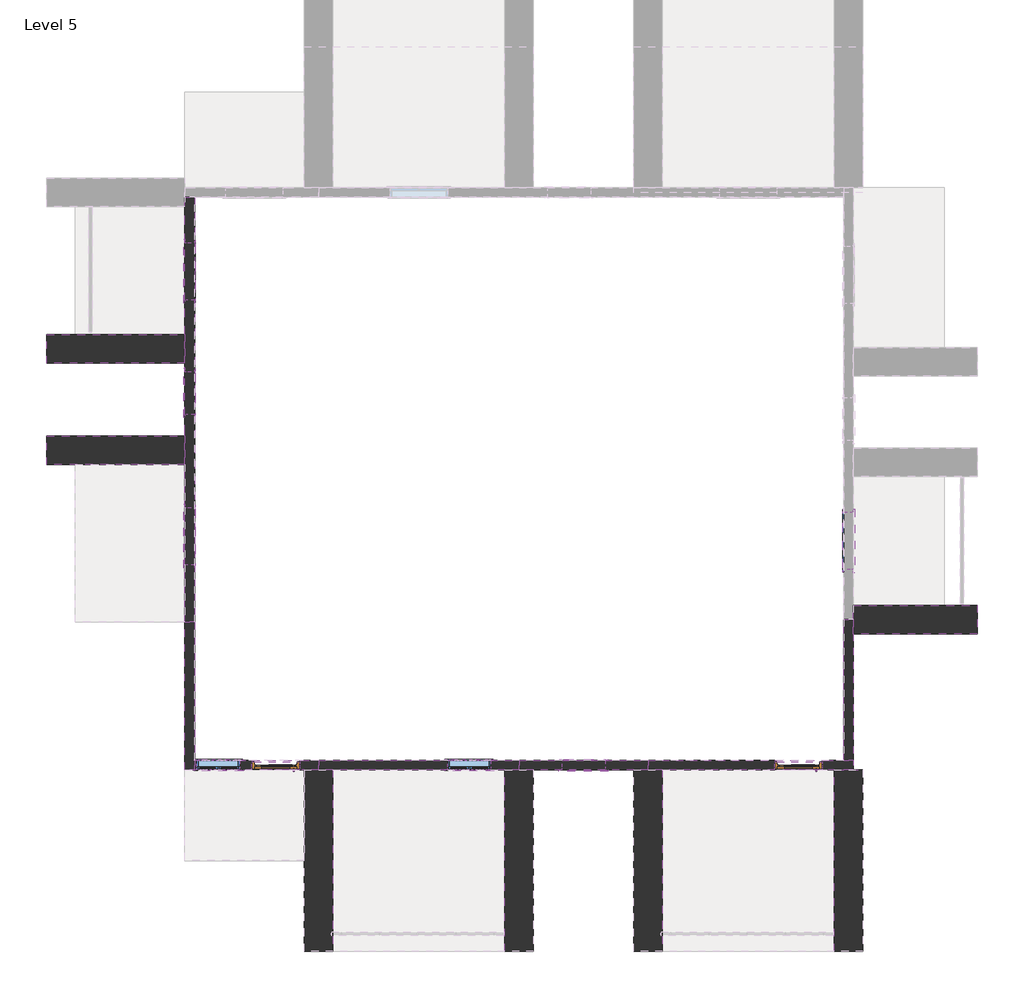
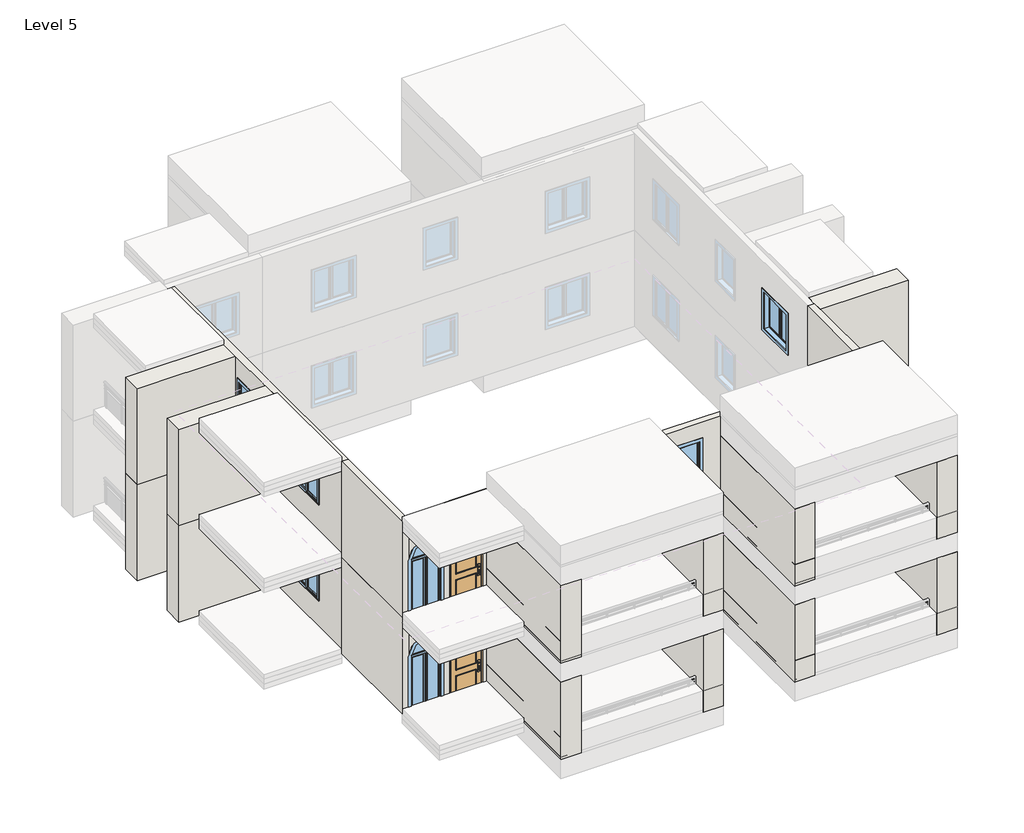
# One storey, part 1 of 4: 28 walls, 14 windows, 4 doors.
"""IFC4 building model written with IfcOpenShell, lengths in millimetres."""

from ifc_helpers import new_model, si_unit, frame, origin, place, context, project, spatial, polyline, circle_curve, outline, extrude, faceted_brep, transform, mapped, element, save
from ifc_brep_helpers import plane_surface, revolved_surface, advanced_brep
from components import door_b6c2ee01, window_4e95f2a8, window_0862ab64, window_8a4441b2

model = new_model("IFC4")

# Units and contexts
model_context = context("Model", 3, world=origin())
ifc_project = project(units=[si_unit("LENGTHUNIT", "METRE", prefix="MILLI")], contexts=[model_context])

# Site, building, storey
site = spatial("IfcSite", under=ifc_project)
building = spatial("IfcBuilding", under=site)
storey = spatial("IfcBuildingStorey", under=building, Name="Level 5", Elevation=12192.0)

# Doors
placement = place(None, origin())
door_shape = door_b6c2ee01(model_context)
element("IfcDoor", 1, ObjectType="Door-Exterior-Single-Two_Lite : 36\" x 94\"", at=placement, inside=storey, context=model_context, shape_type="MappedRepresentation", body=[
    mapped(door_shape, transform((-10452.2937431, -5765.036389, 12192.0), x_axis=(-1.0, 0.0, 0.0), y_axis=(0.0, -1.0, 0.0), z_axis=(0.0, 0.0, 1.0))),
])
element("IfcDoor", 2, ObjectType="Door-Exterior-Single-Two_Lite : 36\" x 94\"", at=placement, inside=storey, context=model_context, shape_type="MappedRepresentation", body=[
    mapped(door_shape, transform((672.9062569, -5765.036389, 12192.0), x_axis=(-1.0, 0.0, 0.0), y_axis=(0.0, -1.0, 0.0), z_axis=(0.0, 0.0, 1.0))),
])
element("IfcDoor", 3, ObjectType="Door-Exterior-Single-Two_Lite : 36\" x 94\"", at=placement, inside=storey, context=model_context, shape_type="MappedRepresentation", body=[
    mapped(door_shape, transform((-10452.2937431, -5765.036389, 15240.0), x_axis=(-1.0, 0.0, 0.0), y_axis=(0.0, -1.0, 0.0), z_axis=(0.0, 0.0, 1.0))),
])
element("IfcDoor", 4, ObjectType="Door-Exterior-Single-Two_Lite : 36\" x 94\"", at=placement, inside=storey, context=model_context, shape_type="MappedRepresentation", body=[
    mapped(door_shape, transform((672.9062569, -5765.036389, 15240.0), x_axis=(-1.0, 0.0, 0.0), y_axis=(0.0, -1.0, 0.0), z_axis=(0.0, 0.0, 1.0))),
])

# Walls
element("IfcWall", 5, ObjectType="Generic - 8\"", at=placement, inside=storey, context=model_context, shape_type="Brep", body=[
    faceted_brep([(-12179.4937431, -5872.986389, 12496.8), (-12179.4937431, -5669.786389, 12496.8), (-12179.4937431, -2723.386389, 12496.8), (-12179.4937431, -2723.386389, 15544.8), (-12179.4937431, -5669.786389, 15544.8), (-12179.4937431, -5872.986389, 15544.8), (-12382.6937431, -5872.986389, 12496.8), (-12382.6937431, -5872.986389, 15544.8), (-12382.6937431, -2723.386389, 15544.8), (-12382.6937431, -2723.386389, 12496.8)], [[[0, 1, 2, 3, 4, 5]], [[6, 7, 8, 9]], [[2, 1, 0, 6, 9]], [[3, 2, 9, 8]], [[5, 4, 3, 8, 7]], [[0, 5, 7, 6]]]),
])
element("IfcWall", 6, ObjectType="Generic - 8\"", at=placement, inside=storey, context=model_context, shape_type="Brep", body=[
    faceted_brep([(-2527.4937431, -5669.786389, 15544.8), (1638.1062569, -5669.786389, 15544.8), (1841.3062569, -5669.786389, 15544.8), (1841.3062569, -5669.786389, 12496.8), (1638.1062569, -5669.786389, 12496.8), (1180.9062569, -5669.786389, 12496.8), (1180.9062569, -5669.786389, 14681.2), (164.9062569, -5669.786389, 14681.2), (164.9062569, -5669.786389, 12496.8), (-2527.4937431, -5669.786389, 12496.8), (1841.3062569, -5872.986389, 15544.8), (-2527.4937431, -5872.986389, 15544.8), (-2527.4937431, -5872.986389, 12496.8), (-2222.6937431, -5872.986389, 12496.8), (164.9062569, -5872.986389, 12496.8), (164.9062569, -5872.986389, 14681.2), (1180.9062569, -5872.986389, 14681.2), (1180.9062569, -5872.986389, 12496.8), (1434.9062569, -5872.986389, 12496.8), (1841.3062569, -5872.986389, 12496.8)], [[[0, 1, 2, 3, 4, 5, 6, 7, 8, 9]], [[10, 11, 12, 13, 14, 15, 16, 17, 18, 19]], [[3, 19, 18, 17, 5, 4]], [[12, 9, 8, 14, 13]], [[2, 1, 0, 11, 10]], [[2, 10, 19, 3]], [[7, 15, 14, 8]], [[15, 7, 6, 16]], [[16, 6, 5, 17]], [[9, 12, 11, 0]]]),
])
element("IfcWall", 7, ObjectType="Generic - 8\"", at=placement, inside=storey, context=model_context, shape_type="Brep", body=[
    faceted_brep([(-12179.4937431, -2723.386389, 12496.8), (-12179.4937431, 6319.013611, 12496.8), (-12179.4937431, 6319.013611, 15544.8), (-12179.4937431, -2723.386389, 15544.8), (-12179.4937431, 2610.613611, 14867.7149116), (-12179.4937431, 2610.613611, 13648.5149116), (-12179.4937431, 1696.213611, 13648.5149116), (-12179.4937431, 1696.213611, 14867.7149116), (-12179.4937431, -284.986389, 14690.8059909), (-12179.4937431, -284.986389, 13471.6059909), (-12179.4937431, -1504.186389, 13471.6059909), (-12179.4937431, -1504.186389, 14690.8059909), (-12179.4937431, 5353.813611, 14617.1335827), (-12179.4937431, 5353.813611, 13397.9335827), (-12179.4937431, 4134.613611, 13397.9335827), (-12179.4937431, 4134.613611, 14617.1335827), (-12382.6937431, -2723.386389, 12496.8), (-12382.6937431, -2723.386389, 15544.8), (-12382.6937431, 629.413611, 15544.8), (-12382.6937431, 1239.013611, 15544.8), (-12382.6937431, 2788.413611, 15544.8), (-12382.6937431, 3398.013611, 15544.8), (-12382.6937431, 6115.813611, 15544.8), (-12382.6937431, 6319.013611, 15544.8), (-12382.6937431, 6319.013611, 12496.8), (-12382.6937431, 6115.813611, 12496.8), (-12382.6937431, 3398.013611, 12496.8), (-12382.6937431, 2788.413611, 12496.8), (-12382.6937431, 1239.013611, 12496.8), (-12382.6937431, 629.413611, 12496.8), (-12382.6937431, 2610.613611, 14867.7149116), (-12382.6937431, 1696.213611, 14867.7149116), (-12382.6937431, 1696.213611, 13648.5149116), (-12382.6937431, 2610.613611, 13648.5149116), (-12382.6937431, -284.986389, 14690.8059909), (-12382.6937431, -1504.186389, 14690.8059909), (-12382.6937431, -1504.186389, 13471.6059909), (-12382.6937431, -284.986389, 13471.6059909), (-12382.6937431, 5353.813611, 14617.1335827), (-12382.6937431, 4134.613611, 14617.1335827), (-12382.6937431, 4134.613611, 13397.9335827), (-12382.6937431, 5353.813611, 13397.9335827)], [[[0, 1, 2, 3], [4, 5, 6, 7], [8, 9, 10, 11], [12, 13, 14, 15]], [[16, 17, 18, 19, 20, 21, 22, 23, 24, 25, 26, 27, 28, 29], [30, 31, 32, 33], [34, 35, 36, 37], [38, 39, 40, 41]], [[1, 0, 16, 29, 28, 27, 26, 25, 24]], [[3, 2, 23, 22, 21, 20, 19, 18, 17]], [[0, 3, 17, 16]], [[2, 1, 24, 23]], [[5, 4, 30, 33]], [[6, 5, 33, 32]], [[7, 6, 32, 31]], [[4, 7, 31, 30]], [[9, 8, 34, 37]], [[10, 9, 37, 36]], [[11, 10, 36, 35]], [[8, 11, 35, 34]], [[13, 12, 38, 41]], [[14, 13, 41, 40]], [[15, 14, 40, 39]], [[12, 15, 39, 38]]]),
])
element("IfcWall", 8, ObjectType="Generic - 8\"", at=placement, inside=storey, context=model_context, shape_type="AdvancedBrep", body=[
    advanced_brep(
    [(-12179.4937431, -5669.786389, 15544.8), (-9537.8937431, -5669.786389, 15544.8), (-9537.8937431, -5669.786389, 12496.8), (-9944.2937431, -5669.786389, 12496.8), (-9944.2937431, -5669.786389, 14681.2), (-10960.2937431, -5669.786389, 14681.2), (-10960.2937431, -5669.786389, 12496.8), (-11214.2937431, -5669.786389, 12496.8), (-11214.2937431, -5669.786389, 14235.597687), (-12128.6937431, -5669.786389, 14235.597687), (-12128.6937431, -5669.786389, 12496.8), (-12179.4937431, -5669.786389, 12496.8), (-9537.8937431, -5872.986389, 15544.8), (-12179.4937431, -5872.986389, 15544.8), (-12179.4937431, -5872.986389, 12496.8), (-12128.6937431, -5872.986389, 12496.8), (-12128.6937431, -5872.986389, 14235.597687), (-11214.2937431, -5872.986389, 14235.597687), (-11214.2937431, -5872.986389, 12496.8), (-10960.2937431, -5872.986389, 12496.8), (-10960.2937431, -5872.986389, 14681.2), (-9944.2937431, -5872.986389, 14681.2), (-9944.2937431, -5872.986389, 12496.8), (-9842.6937431, -5872.986389, 12496.8), (-9537.8937431, -5872.986389, 12496.8)],
    [
        (0, 1),
        (1, 2),
        (2, 3),
        (3, 4),
        (4, 5),
        (5, 6),
        (6, 7),
        (7, 8),
        (8, 9, circle_curve(frame((-11671.4937431, -5669.786389, 14235.597687), z_axis=(0.0, -1.0, 0.0), x_axis=(-1.0, 0.0, 0.0)), 457.2)),
        (9, 10),
        (10, 11),
        (11, 0),
        (12, 13),
        (13, 14),
        (14, 15),
        (15, 16),
        (16, 17, circle_curve(frame((-11671.4937431, -5872.986389, 14235.597687), z_axis=(0.0, 1.0, 0.0), x_axis=(-1.0, 0.0, 0.0)), 457.2)),
        (17, 18),
        (18, 19),
        (19, 20),
        (20, 21),
        (21, 22),
        (22, 23),
        (23, 24),
        (24, 12),
        (14, 11),
        (10, 15),
        (2, 24),
        (22, 3),
        (6, 19),
        (18, 7),
        (0, 13),
        (12, 1),
        (5, 20),
        (4, 21),
        (9, 16),
        (17, 8),
    ],
    [
        plane_surface(frame((1423.3958892, -5669.786389, 12496.8), z_axis=(0.0, 1.0, 0.0), x_axis=(-1.0, 0.0, 0.0))),
        plane_surface(frame((1423.3958892, -5872.986389, 12496.8), z_axis=(0.0, -1.0, 0.0), x_axis=(1.0, 0.0, 0.0))),
        plane_surface(frame((-9537.8937431, -5669.786389, 12496.8), z_axis=(0.0, 0.0, -1.0), x_axis=(0.0, -1.0, 0.0))),
        plane_surface(frame((-12281.0937431, -5669.786389, 15544.8), z_axis=(0.0, 0.0, 1.0), x_axis=(0.0, -1.0, 0.0))),
        plane_surface(frame((-12179.4937431, 6416.9740134, 12496.8), z_axis=(-1.0, 0.0, 0.0), x_axis=(0.0, 1.0, 0.0))),
        plane_surface(frame((-9537.8937431, -5669.786389, 15544.8), z_axis=(1.0, 0.0, 0.0), x_axis=(0.0, -1.0, 0.0))),
        plane_surface(frame((-10960.2937431, -4145.786389, 12192.0), z_axis=(1.0, 0.0, 0.0), x_axis=(0.0, -1.0, 0.0))),
        plane_surface(frame((-10960.2937431, -4145.786389, 14681.2), z_axis=(0.0, 0.0, -1.0), x_axis=(0.0, -1.0, 0.0))),
        plane_surface(frame((-9944.2937431, -4145.786389, 14681.2), z_axis=(-1.0, 0.0, 0.0), x_axis=(0.0, -1.0, 0.0))),
        plane_surface(frame((-12128.6937431, -7193.786389, 14235.597687), z_axis=(1.0, 0.0, 0.0), x_axis=(0.0, 1.0, 0.0))),
        plane_surface(frame((-11214.2937431, -7193.786389, 12387.747687), z_axis=(-1.0, 0.0, 0.0), x_axis=(0.0, 1.0, 0.0))),
        revolved_surface(polyline([(-12128.6937431, -5872.986389, 14235.597687), (-12128.6937431, -5669.786389, 14235.597687)]), (-11671.4937431, -4145.786389, 14235.597687), (0.0, -1.0, 0.0)),
    ],
    [
        (0, [[1, 2, 3, 4, 5, 6, 7, 8, 9, 10, 11, 12]]),
        (1, [[13, 14, 15, 16, 17, 18, 19, 20, 21, 22, 23, 24, 25]]),
        (2, [[26, -11, 27, -15]]),
        (2, [[28, -24, -23, 29, -3]]),
        (2, [[30, -19, 31, -7]]),
        (3, [[-1, 32, -13, 33]]),
        (4, [[-12, -26, -14, -32]]),
        (5, [[-33, -25, -28, -2]]),
        (6, [[34, -20, -30, -6]]),
        (7, [[-34, -5, 35, -21]]),
        (8, [[-35, -4, -29, -22]]),
        (9, [[36, -16, -27, -10]]),
        (10, [[37, -8, -31, -18]]),
        (11, [[-36, -9, -37, -17]]),
    ],
),
])
element("IfcWall", 9, ObjectType="Generic - 8\"", at=placement, inside=storey, context=model_context, shape_type="Brep", body=[
    faceted_brep([(1638.1062569, -2672.586389, 12496.8), (1638.1062569, -5669.786389, 12496.8), (1638.1062569, -5669.786389, 15544.8), (1638.1062569, -2672.586389, 15544.8), (1841.3062569, -2672.586389, 12496.8), (1841.3062569, -2672.586389, 15544.8), (1841.3062569, -2977.386389, 15544.8), (1841.3062569, -5669.786389, 15544.8), (1841.3062569, -5669.786389, 12496.8), (1841.3062569, -2977.386389, 12496.8)], [[[0, 1, 2, 3]], [[4, 5, 6, 7, 8, 9]], [[1, 0, 4, 9, 8]], [[3, 2, 7, 6, 5]], [[0, 3, 5, 4]], [[1, 8, 7, 2]]]),
])
element("IfcWall", 10, ObjectType="Generic - 8\"", at=placement, inside=storey, context=model_context, shape_type="Brep", body=[
    faceted_brep([(-2527.4937431, -5669.786389, 15544.8), (-2527.4937431, -5669.786389, 12496.8), (-5270.6937431, -5669.786389, 12496.8), (-5270.6937431, -5669.786389, 15544.8), (-4356.2937431, -5669.786389, 14991.074951), (-4356.2937431, -5669.786389, 13771.874951), (-3441.8937431, -5669.786389, 13771.874951), (-3441.8937431, -5669.786389, 14991.074951), (-2527.4937431, -5872.986389, 12496.8), (-2527.4937431, -5872.986389, 15544.8), (-5270.6937431, -5872.986389, 15544.8), (-5270.6937431, -5872.986389, 12496.8), (-4965.8937431, -5872.986389, 12496.8), (-2832.2937431, -5872.986389, 12496.8), (-4356.2937431, -5872.986389, 14991.074951), (-3441.8937431, -5872.986389, 14991.074951), (-3441.8937431, -5872.986389, 13771.874951), (-4356.2937431, -5872.986389, 13771.874951)], [[[0, 1, 2, 3], [4, 5, 6, 7]], [[8, 9, 10, 11, 12, 13], [14, 15, 16, 17]], [[2, 1, 8, 13, 12, 11]], [[0, 3, 10, 9]], [[5, 4, 14, 17]], [[6, 5, 17, 16]], [[7, 6, 16, 15]], [[4, 7, 15, 14]], [[0, 9, 8, 1]], [[2, 11, 10, 3]]]),
])
element("IfcWall", 11, ObjectType="Generic - 8\"", at=placement, inside=storey, context=model_context, shape_type="AdvancedBrep", body=[
    advanced_brep(
    [(-9537.8937431, -5669.786389, 15544.8), (-5270.6937431, -5669.786389, 15544.8), (-5270.6937431, -5669.786389, 12496.8), (-5880.2937431, -5669.786389, 12496.8), (-5880.2937431, -5669.786389, 14192.25), (-6794.6937431, -5669.786389, 14192.25), (-6794.6937431, -5669.786389, 12496.8), (-9537.8937431, -5669.786389, 12496.8), (-5270.6937431, -5872.986389, 15544.8), (-9537.8937431, -5872.986389, 15544.8), (-9537.8937431, -5872.986389, 12496.8), (-9233.0937431, -5872.986389, 12496.8), (-6794.6937431, -5872.986389, 12496.8), (-6794.6937431, -5872.986389, 14192.25), (-5880.2937431, -5872.986389, 14192.25), (-5880.2937431, -5872.986389, 12496.8), (-5575.4937431, -5872.986389, 12496.8), (-5270.6937431, -5872.986389, 12496.8)],
    [
        (0, 1),
        (1, 2),
        (2, 3),
        (3, 4),
        (4, 5, circle_curve(frame((-6337.4937431, -5669.786389, 14192.25), z_axis=(0.0, -1.0, 0.0), x_axis=(-1.0, 0.0, 0.0)), 457.2)),
        (5, 6),
        (6, 7),
        (7, 0),
        (8, 9),
        (9, 10),
        (10, 11),
        (11, 12),
        (12, 13),
        (13, 14, circle_curve(frame((-6337.4937431, -5872.986389, 14192.25), z_axis=(0.0, 1.0, 0.0), x_axis=(-1.0, 0.0, 0.0)), 457.2)),
        (14, 15),
        (15, 16),
        (16, 17),
        (17, 8),
        (10, 7),
        (6, 12),
        (2, 17),
        (15, 3),
        (0, 9),
        (8, 1),
        (5, 13),
        (14, 4),
    ],
    [
        plane_surface(frame((1423.3958892, -5669.786389, 12496.8), z_axis=(0.0, 1.0, 0.0), x_axis=(-1.0, 0.0, 0.0))),
        plane_surface(frame((1423.3958892, -5872.986389, 12496.8), z_axis=(0.0, -1.0, 0.0), x_axis=(1.0, 0.0, 0.0))),
        plane_surface(frame((-5270.6937431, -5669.786389, 12496.8), z_axis=(0.0, 0.0, -1.0), x_axis=(0.0, -1.0, 0.0))),
        plane_surface(frame((-9537.8937431, -5669.786389, 15544.8), z_axis=(0.0, 0.0, 1.0), x_axis=(0.0, -1.0, 0.0))),
        plane_surface(frame((-6794.6937431, -7193.786389, 14192.25), z_axis=(1.0, 0.0, 0.0), x_axis=(0.0, 1.0, 0.0))),
        plane_surface(frame((-5880.2937431, -7193.786389, 12344.4), z_axis=(-1.0, 0.0, 0.0), x_axis=(0.0, 1.0, 0.0))),
        revolved_surface(polyline([(-6794.6937431, -5872.986389, 14192.25), (-6794.6937431, -5669.786389, 14192.25)]), (-6337.4937431, -4145.786389, 14192.25), (0.0, -1.0, 0.0)),
        plane_surface(frame((-5270.6937431, -5669.786389, 15544.8), z_axis=(1.0, 0.0, 0.0), x_axis=(0.0, -1.0, 0.0))),
        plane_surface(frame((-9537.8937431, -5669.786389, 12496.8), z_axis=(-1.0, 0.0, 0.0), x_axis=(0.0, -1.0, 0.0))),
    ],
    [
        (0, [[1, 2, 3, 4, 5, 6, 7, 8]]),
        (1, [[9, 10, 11, 12, 13, 14, 15, 16, 17, 18]]),
        (2, [[19, -7, 20, -12, -11]]),
        (2, [[21, -17, -16, 22, -3]]),
        (3, [[-1, 23, -9, 24]]),
        (4, [[25, -13, -20, -6]]),
        (5, [[26, -4, -22, -15]]),
        (6, [[-25, -5, -26, -14]]),
        (7, [[-24, -18, -21, -2]]),
        (8, [[-19, -10, -23, -8]]),
    ],
),
])
element("IfcWall", 12, ObjectType="Generic - 8\"", at=placement, inside=storey, context=model_context, shape_type="Brep", body=[
    faceted_brep([(-12179.4937431, -5872.986389, 15544.8), (-12179.4937431, -5669.786389, 15544.8), (-12179.4937431, -2723.386389, 15544.8), (-12179.4937431, -2723.386389, 18592.8), (-12179.4937431, -5669.786389, 18592.8), (-12179.4937431, -5872.986389, 18592.8), (-12382.6937431, -5872.986389, 15544.8), (-12382.6937431, -5872.986389, 18592.8), (-12382.6937431, -2723.386389, 18592.8), (-12382.6937431, -2723.386389, 15544.8)], [[[0, 1, 2, 3, 4, 5]], [[6, 7, 8, 9]], [[2, 1, 0, 6, 9]], [[3, 2, 9, 8]], [[5, 4, 3, 8, 7]], [[0, 5, 7, 6]]]),
])
element("IfcWall", 13, ObjectType="Generic - 8\"", at=placement, inside=storey, context=model_context, shape_type="Brep", body=[
    faceted_brep([(-2527.4937431, -5669.786389, 18592.8), (1638.1062569, -5669.786389, 18592.8), (1841.3062569, -5669.786389, 18592.8), (1841.3062569, -5669.786389, 15544.8), (1638.1062569, -5669.786389, 15544.8), (1180.9062569, -5669.786389, 15544.8), (1180.9062569, -5669.786389, 17729.2), (164.9062569, -5669.786389, 17729.2), (164.9062569, -5669.786389, 15544.8), (-2527.4937431, -5669.786389, 15544.8), (1841.3062569, -5872.986389, 18592.8), (-2527.4937431, -5872.986389, 18592.8), (-2527.4937431, -5872.986389, 15544.8), (-2222.6937431, -5872.986389, 15544.8), (164.9062569, -5872.986389, 15544.8), (164.9062569, -5872.986389, 17729.2), (1180.9062569, -5872.986389, 17729.2), (1180.9062569, -5872.986389, 15544.8), (1434.9062569, -5872.986389, 15544.8), (1841.3062569, -5872.986389, 15544.8)], [[[0, 1, 2, 3, 4, 5, 6, 7, 8, 9]], [[10, 11, 12, 13, 14, 15, 16, 17, 18, 19]], [[3, 19, 18, 17, 5, 4]], [[12, 9, 8, 14, 13]], [[2, 1, 0, 11, 10]], [[2, 10, 19, 3]], [[7, 15, 14, 8]], [[15, 7, 6, 16]], [[16, 6, 5, 17]], [[9, 12, 11, 0]]]),
])
element("IfcWall", 14, ObjectType="Generic - 8\"", at=placement, inside=storey, context=model_context, shape_type="Brep", body=[
    faceted_brep([(-12179.4937431, -2723.386389, 15544.8), (-12179.4937431, 6319.013611, 15544.8), (-12179.4937431, 6319.013611, 18592.8), (-12179.4937431, -2723.386389, 18592.8), (-12179.4937431, 2610.613611, 17915.7149116), (-12179.4937431, 2610.613611, 16696.5149116), (-12179.4937431, 1696.213611, 16696.5149116), (-12179.4937431, 1696.213611, 17915.7149116), (-12179.4937431, -284.986389, 17738.8059909), (-12179.4937431, -284.986389, 16519.6059909), (-12179.4937431, -1504.186389, 16519.6059909), (-12179.4937431, -1504.186389, 17738.8059909), (-12179.4937431, 5353.813611, 17665.1335827), (-12179.4937431, 5353.813611, 16445.9335827), (-12179.4937431, 4134.613611, 16445.9335827), (-12179.4937431, 4134.613611, 17665.1335827), (-12382.6937431, -2723.386389, 15544.8), (-12382.6937431, -2723.386389, 18592.8), (-12382.6937431, 629.413611, 18592.8), (-12382.6937431, 1239.013611, 18592.8), (-12382.6937431, 2788.413611, 18592.8), (-12382.6937431, 3398.013611, 18592.8), (-12382.6937431, 6115.813611, 18592.8), (-12382.6937431, 6319.013611, 18592.8), (-12382.6937431, 6319.013611, 15544.8), (-12382.6937431, 6115.813611, 15544.8), (-12382.6937431, 3398.013611, 15544.8), (-12382.6937431, 2788.413611, 15544.8), (-12382.6937431, 1239.013611, 15544.8), (-12382.6937431, 629.413611, 15544.8), (-12382.6937431, 2610.613611, 17915.7149116), (-12382.6937431, 1696.213611, 17915.7149116), (-12382.6937431, 1696.213611, 16696.5149116), (-12382.6937431, 2610.613611, 16696.5149116), (-12382.6937431, -284.986389, 17738.8059909), (-12382.6937431, -1504.186389, 17738.8059909), (-12382.6937431, -1504.186389, 16519.6059909), (-12382.6937431, -284.986389, 16519.6059909), (-12382.6937431, 5353.813611, 17665.1335827), (-12382.6937431, 4134.613611, 17665.1335827), (-12382.6937431, 4134.613611, 16445.9335827), (-12382.6937431, 5353.813611, 16445.9335827)], [[[0, 1, 2, 3], [4, 5, 6, 7], [8, 9, 10, 11], [12, 13, 14, 15]], [[16, 17, 18, 19, 20, 21, 22, 23, 24, 25, 26, 27, 28, 29], [30, 31, 32, 33], [34, 35, 36, 37], [38, 39, 40, 41]], [[1, 0, 16, 29, 28, 27, 26, 25, 24]], [[3, 2, 23, 22, 21, 20, 19, 18, 17]], [[0, 3, 17, 16]], [[2, 1, 24, 23]], [[5, 4, 30, 33]], [[6, 5, 33, 32]], [[7, 6, 32, 31]], [[4, 7, 31, 30]], [[9, 8, 34, 37]], [[10, 9, 37, 36]], [[11, 10, 36, 35]], [[8, 11, 35, 34]], [[13, 12, 38, 41]], [[14, 13, 41, 40]], [[15, 14, 40, 39]], [[12, 15, 39, 38]]]),
])
element("IfcWall", 15, ObjectType="Generic - 8\"", at=placement, inside=storey, context=model_context, shape_type="AdvancedBrep", body=[
    advanced_brep(
    [(-12179.4937431, -5669.786389, 18592.8), (-9537.8937431, -5669.786389, 18592.8), (-9537.8937431, -5669.786389, 15544.8), (-9944.2937431, -5669.786389, 15544.8), (-9944.2937431, -5669.786389, 17729.2), (-10960.2937431, -5669.786389, 17729.2), (-10960.2937431, -5669.786389, 15544.8), (-11214.2937431, -5669.786389, 15544.8), (-11214.2937431, -5669.786389, 17283.597687), (-12128.6937431, -5669.786389, 17283.597687), (-12128.6937431, -5669.786389, 15544.8), (-12179.4937431, -5669.786389, 15544.8), (-9537.8937431, -5872.986389, 18592.8), (-12179.4937431, -5872.986389, 18592.8), (-12179.4937431, -5872.986389, 15544.8), (-12128.6937431, -5872.986389, 15544.8), (-12128.6937431, -5872.986389, 17283.597687), (-11214.2937431, -5872.986389, 17283.597687), (-11214.2937431, -5872.986389, 15544.8), (-10960.2937431, -5872.986389, 15544.8), (-10960.2937431, -5872.986389, 17729.2), (-9944.2937431, -5872.986389, 17729.2), (-9944.2937431, -5872.986389, 15544.8), (-9842.6937431, -5872.986389, 15544.8), (-9537.8937431, -5872.986389, 15544.8)],
    [
        (0, 1),
        (1, 2),
        (2, 3),
        (3, 4),
        (4, 5),
        (5, 6),
        (6, 7),
        (7, 8),
        (8, 9, circle_curve(frame((-11671.4937431, -5669.786389, 17283.597687), z_axis=(0.0, -1.0, 0.0), x_axis=(-1.0, 0.0, 0.0)), 457.2)),
        (9, 10),
        (10, 11),
        (11, 0),
        (12, 13),
        (13, 14),
        (14, 15),
        (15, 16),
        (16, 17, circle_curve(frame((-11671.4937431, -5872.986389, 17283.597687), z_axis=(0.0, 1.0, 0.0), x_axis=(-1.0, 0.0, 0.0)), 457.2)),
        (17, 18),
        (18, 19),
        (19, 20),
        (20, 21),
        (21, 22),
        (22, 23),
        (23, 24),
        (24, 12),
        (14, 11),
        (10, 15),
        (2, 24),
        (22, 3),
        (6, 19),
        (18, 7),
        (0, 13),
        (12, 1),
        (5, 20),
        (4, 21),
        (9, 16),
        (17, 8),
    ],
    [
        plane_surface(frame((1423.3958892, -5669.786389, 15544.8), z_axis=(0.0, 1.0, 0.0), x_axis=(-1.0, 0.0, 0.0))),
        plane_surface(frame((1423.3958892, -5872.986389, 15544.8), z_axis=(0.0, -1.0, 0.0), x_axis=(1.0, 0.0, 0.0))),
        plane_surface(frame((-9537.8937431, -5669.786389, 15544.8), z_axis=(0.0, 0.0, -1.0), x_axis=(0.0, -1.0, 0.0))),
        plane_surface(frame((-12281.0937431, -5669.786389, 18592.8), z_axis=(0.0, 0.0, 1.0), x_axis=(0.0, -1.0, 0.0))),
        plane_surface(frame((-12179.4937431, 6416.9740134, 15544.8), z_axis=(-1.0, 0.0, 0.0), x_axis=(0.0, 1.0, 0.0))),
        plane_surface(frame((-9537.8937431, -5669.786389, 18592.8), z_axis=(1.0, 0.0, 0.0), x_axis=(0.0, -1.0, 0.0))),
        plane_surface(frame((-10960.2937431, -4145.786389, 15240.0), z_axis=(1.0, 0.0, 0.0), x_axis=(0.0, -1.0, 0.0))),
        plane_surface(frame((-10960.2937431, -4145.786389, 17729.2), z_axis=(0.0, 0.0, -1.0), x_axis=(0.0, -1.0, 0.0))),
        plane_surface(frame((-9944.2937431, -4145.786389, 17729.2), z_axis=(-1.0, 0.0, 0.0), x_axis=(0.0, -1.0, 0.0))),
        plane_surface(frame((-12128.6937431, -7193.786389, 17283.597687), z_axis=(1.0, 0.0, 0.0), x_axis=(0.0, 1.0, 0.0))),
        plane_surface(frame((-11214.2937431, -7193.786389, 15435.747687), z_axis=(-1.0, 0.0, 0.0), x_axis=(0.0, 1.0, 0.0))),
        revolved_surface(polyline([(-12128.6937431, -5872.986389, 17283.597687), (-12128.6937431, -5669.786389, 17283.597687)]), (-11671.4937431, -4145.786389, 17283.597687), (0.0, -1.0, 0.0)),
    ],
    [
        (0, [[1, 2, 3, 4, 5, 6, 7, 8, 9, 10, 11, 12]]),
        (1, [[13, 14, 15, 16, 17, 18, 19, 20, 21, 22, 23, 24, 25]]),
        (2, [[26, -11, 27, -15]]),
        (2, [[28, -24, -23, 29, -3]]),
        (2, [[30, -19, 31, -7]]),
        (3, [[-1, 32, -13, 33]]),
        (4, [[-12, -26, -14, -32]]),
        (5, [[-33, -25, -28, -2]]),
        (6, [[34, -20, -30, -6]]),
        (7, [[-34, -5, 35, -21]]),
        (8, [[-35, -4, -29, -22]]),
        (9, [[36, -16, -27, -10]]),
        (10, [[37, -8, -31, -18]]),
        (11, [[-36, -9, -37, -17]]),
    ],
),
])
element("IfcWall", 16, ObjectType="Generic - 8\"", at=placement, inside=storey, context=model_context, shape_type="Brep", body=[
    faceted_brep([(1638.1062569, -2672.586389, 15544.8), (1638.1062569, -5669.786389, 15544.8), (1638.1062569, -5669.786389, 18592.8), (1638.1062569, -2672.586389, 18592.8), (1841.3062569, -2672.586389, 15544.8), (1841.3062569, -2672.586389, 18592.8), (1841.3062569, -2977.386389, 18592.8), (1841.3062569, -5669.786389, 18592.8), (1841.3062569, -5669.786389, 15544.8), (1841.3062569, -2977.386389, 15544.8)], [[[0, 1, 2, 3]], [[4, 5, 6, 7, 8, 9]], [[1, 0, 4, 9, 8]], [[3, 2, 7, 6, 5]], [[0, 3, 5, 4]], [[1, 8, 7, 2]]]),
])
element("IfcWall", 17, ObjectType="Generic - 8\"", at=placement, inside=storey, context=model_context, shape_type="Brep", body=[
    faceted_brep([(-2527.4937431, -5669.786389, 18592.8), (-2527.4937431, -5669.786389, 15544.8), (-5270.6937431, -5669.786389, 15544.8), (-5270.6937431, -5669.786389, 18592.8), (-4356.2937431, -5669.786389, 18039.074951), (-4356.2937431, -5669.786389, 16819.874951), (-3441.8937431, -5669.786389, 16819.874951), (-3441.8937431, -5669.786389, 18039.074951), (-2527.4937431, -5872.986389, 15544.8), (-2527.4937431, -5872.986389, 18592.8), (-5270.6937431, -5872.986389, 18592.8), (-5270.6937431, -5872.986389, 15544.8), (-4965.8937431, -5872.986389, 15544.8), (-2832.2937431, -5872.986389, 15544.8), (-4356.2937431, -5872.986389, 18039.074951), (-3441.8937431, -5872.986389, 18039.074951), (-3441.8937431, -5872.986389, 16819.874951), (-4356.2937431, -5872.986389, 16819.874951)], [[[0, 1, 2, 3], [4, 5, 6, 7]], [[8, 9, 10, 11, 12, 13], [14, 15, 16, 17]], [[2, 1, 8, 13, 12, 11]], [[0, 3, 10, 9]], [[5, 4, 14, 17]], [[6, 5, 17, 16]], [[7, 6, 16, 15]], [[4, 7, 15, 14]], [[0, 9, 8, 1]], [[2, 11, 10, 3]]]),
])
element("IfcWall", 18, ObjectType="Generic - 8\"", at=placement, inside=storey, context=model_context, shape_type="AdvancedBrep", body=[
    advanced_brep(
    [(-9537.8937431, -5669.786389, 18592.8), (-5270.6937431, -5669.786389, 18592.8), (-5270.6937431, -5669.786389, 15544.8), (-5880.2937431, -5669.786389, 15544.8), (-5880.2937431, -5669.786389, 17240.25), (-6794.6937431, -5669.786389, 17240.25), (-6794.6937431, -5669.786389, 15544.8), (-9537.8937431, -5669.786389, 15544.8), (-5270.6937431, -5872.986389, 18592.8), (-9537.8937431, -5872.986389, 18592.8), (-9537.8937431, -5872.986389, 15544.8), (-9233.0937431, -5872.986389, 15544.8), (-6794.6937431, -5872.986389, 15544.8), (-6794.6937431, -5872.986389, 17240.25), (-5880.2937431, -5872.986389, 17240.25), (-5880.2937431, -5872.986389, 15544.8), (-5575.4937431, -5872.986389, 15544.8), (-5270.6937431, -5872.986389, 15544.8)],
    [
        (0, 1),
        (1, 2),
        (2, 3),
        (3, 4),
        (4, 5, circle_curve(frame((-6337.4937431, -5669.786389, 17240.25), z_axis=(0.0, -1.0, 0.0), x_axis=(-1.0, 0.0, 0.0)), 457.2)),
        (5, 6),
        (6, 7),
        (7, 0),
        (8, 9),
        (9, 10),
        (10, 11),
        (11, 12),
        (12, 13),
        (13, 14, circle_curve(frame((-6337.4937431, -5872.986389, 17240.25), z_axis=(0.0, 1.0, 0.0), x_axis=(-1.0, 0.0, 0.0)), 457.2)),
        (14, 15),
        (15, 16),
        (16, 17),
        (17, 8),
        (10, 7),
        (6, 12),
        (2, 17),
        (15, 3),
        (0, 9),
        (8, 1),
        (5, 13),
        (14, 4),
    ],
    [
        plane_surface(frame((1423.3958892, -5669.786389, 15544.8), z_axis=(0.0, 1.0, 0.0), x_axis=(-1.0, 0.0, 0.0))),
        plane_surface(frame((1423.3958892, -5872.986389, 15544.8), z_axis=(0.0, -1.0, 0.0), x_axis=(1.0, 0.0, 0.0))),
        plane_surface(frame((-5270.6937431, -5669.786389, 15544.8), z_axis=(0.0, 0.0, -1.0), x_axis=(0.0, -1.0, 0.0))),
        plane_surface(frame((-9537.8937431, -5669.786389, 18592.8), z_axis=(0.0, 0.0, 1.0), x_axis=(0.0, -1.0, 0.0))),
        plane_surface(frame((-6794.6937431, -7193.786389, 17240.25), z_axis=(1.0, 0.0, 0.0), x_axis=(0.0, 1.0, 0.0))),
        plane_surface(frame((-5880.2937431, -7193.786389, 15392.4), z_axis=(-1.0, 0.0, 0.0), x_axis=(0.0, 1.0, 0.0))),
        revolved_surface(polyline([(-6794.6937431, -5872.986389, 17240.25), (-6794.6937431, -5669.786389, 17240.25)]), (-6337.4937431, -4145.786389, 17240.25), (0.0, -1.0, 0.0)),
        plane_surface(frame((-5270.6937431, -5669.786389, 18592.8), z_axis=(1.0, 0.0, 0.0), x_axis=(0.0, -1.0, 0.0))),
        plane_surface(frame((-9537.8937431, -5669.786389, 15544.8), z_axis=(-1.0, 0.0, 0.0), x_axis=(0.0, -1.0, 0.0))),
    ],
    [
        (0, [[1, 2, 3, 4, 5, 6, 7, 8]]),
        (1, [[9, 10, 11, 12, 13, 14, 15, 16, 17, 18]]),
        (2, [[19, -7, 20, -12, -11]]),
        (2, [[21, -17, -16, 22, -3]]),
        (3, [[-1, 23, -9, 24]]),
        (4, [[25, -13, -20, -6]]),
        (5, [[26, -4, -22, -15]]),
        (6, [[-25, -5, -26, -14]]),
        (7, [[-24, -18, -21, -2]]),
        (8, [[-19, -10, -23, -8]]),
    ],
),
])
element("IfcWall", 19, ObjectType="Generic -2' 2", at=placement, inside=storey, context=model_context, shape_type="SweptSolid", body=[
    extrude(outline(polyline([(-15329.0937431, 3398.013611), (-12382.6937431, 3398.013611), (-12382.6937431, 2788.413611), (-15329.0937431, 2788.413611), (-15329.0937431, 3398.013611)])), frame((0.0, 0.0, 12496.8), z_axis=(0.0, 0.0, 1.0), x_axis=(1.0, 0.0, 0.0)), (0.0, 0.0, 1.0), 3048.0),
])
element("IfcWall", 20, ObjectType="Generic -2' 2", at=placement, inside=storey, context=model_context, shape_type="SweptSolid", body=[
    extrude(outline(polyline([(-15329.0937431, 1239.013611), (-12382.6937431, 1239.013611), (-12382.6937431, 629.413611), (-15329.0937431, 629.413611), (-15329.0937431, 1239.013611)])), frame((0.0, 0.0, 12496.8), z_axis=(0.0, 0.0, 1.0), x_axis=(1.0, 0.0, 0.0)), (0.0, 0.0, 1.0), 3048.0),
])
element("IfcWall", 21, ObjectType="Generic -2' 2", at=placement, inside=storey, context=model_context, shape_type="Brep", body=[
    faceted_brep([(1841.3062569, -2977.386389, 12496.8), (4482.9062569, -2977.386389, 12496.8), (4482.9062569, -2977.386389, 15544.8), (1841.3062569, -2977.386389, 15544.8), (1841.3062569, -2367.786389, 12496.8), (1841.3062569, -2367.786389, 15544.8), (4482.9062569, -2367.786389, 15544.8), (4482.9062569, -2367.786389, 12496.8), (1841.3062569, -2672.586389, 12496.8), (1841.3062569, -2672.586389, 15544.8)], [[[0, 1, 2, 3]], [[4, 5, 6, 7]], [[1, 0, 8, 4, 7]], [[2, 1, 7, 6]], [[3, 2, 6, 5, 9]], [[0, 3, 9, 5, 4, 8]]]),
])
element("IfcWall", 22, ObjectType="Generic -2' 2", at=placement, inside=storey, context=model_context, shape_type="SweptSolid", body=[
    extrude(outline(polyline([(-15329.0937431, 3398.013611), (-12382.6937431, 3398.013611), (-12382.6937431, 2788.413611), (-15329.0937431, 2788.413611), (-15329.0937431, 3398.013611)])), frame((0.0, 0.0, 15544.8), z_axis=(0.0, 0.0, 1.0), x_axis=(1.0, 0.0, 0.0)), (0.0, 0.0, 1.0), 3048.0),
])
element("IfcWall", 23, ObjectType="Generic -2' 2", at=placement, inside=storey, context=model_context, shape_type="SweptSolid", body=[
    extrude(outline(polyline([(-15329.0937431, 1239.013611), (-12382.6937431, 1239.013611), (-12382.6937431, 629.413611), (-15329.0937431, 629.413611), (-15329.0937431, 1239.013611)])), frame((0.0, 0.0, 15544.8), z_axis=(0.0, 0.0, 1.0), x_axis=(1.0, 0.0, 0.0)), (0.0, 0.0, 1.0), 3048.0),
])
element("IfcWall", 24, ObjectType="Generic -2' 2", at=placement, inside=storey, context=model_context, shape_type="Brep", body=[
    faceted_brep([(1841.3062569, -2977.386389, 15544.8), (4482.9062569, -2977.386389, 15544.8), (4482.9062569, -2977.386389, 18592.8), (1841.3062569, -2977.386389, 18592.8), (1841.3062569, -2367.786389, 15544.8), (1841.3062569, -2367.786389, 18592.8), (4482.9062569, -2367.786389, 18592.8), (4482.9062569, -2367.786389, 15544.8), (1841.3062569, -2672.586389, 15544.8), (1841.3062569, -2672.586389, 18592.8)], [[[0, 1, 2, 3]], [[4, 5, 6, 7]], [[1, 0, 8, 4, 7]], [[2, 1, 7, 6]], [[3, 2, 6, 5, 9]], [[0, 3, 9, 5, 4, 8]]]),
])
element("IfcWall", 25, ObjectType="Generic -2' 3 red", at=placement, inside=storey, context=model_context, shape_type="Brep", body=[
    faceted_brep([(1434.9062569, -5872.986389, 12496.8), (1434.9062569, -9733.786389, 12496.8), (1434.9062569, -9733.786389, 14935.2), (1434.9062569, -5872.986389, 14935.2), (2044.5062569, -5872.986389, 12496.8), (2044.5062569, -5872.986389, 14935.2), (2044.5062569, -9733.786389, 14935.2), (2044.5062569, -9733.786389, 12496.8), (1841.3062569, -5872.986389, 12496.8)], [[[0, 1, 2, 3]], [[4, 5, 6, 7]], [[1, 0, 8, 4, 7]], [[2, 1, 7, 6]], [[3, 2, 6, 5]], [[0, 3, 5, 4, 8]]]),
])
element("IfcWall", 26, ObjectType="Generic -2' 3 red", at=placement, inside=storey, context=model_context, shape_type="Brep", body=[
    faceted_brep([(-2832.2937431, -5872.986389, 12496.8), (-2832.2937431, -9733.786389, 12496.8), (-2832.2937431, -9733.786389, 14942.8571637), (-2832.2937431, -5872.986389, 14942.8571637), (-2222.6937431, -5872.986389, 12496.8), (-2222.6937431, -5872.986389, 14942.8571637), (-2222.6937431, -9733.786389, 14942.8571637), (-2222.6937431, -9733.786389, 12496.8), (-2527.4937431, -5872.986389, 12496.8)], [[[0, 1, 2, 3]], [[4, 5, 6, 7]], [[1, 0, 8, 4, 7]], [[2, 1, 7, 6]], [[3, 2, 6, 5]], [[0, 3, 5, 4, 8]]]),
])
element("IfcWall", 27, ObjectType="Generic -2' 3 red", at=placement, inside=storey, context=model_context, shape_type="Brep", body=[
    faceted_brep([(-5575.4937431, -5872.986389, 12496.8), (-5575.4937431, -9733.786389, 12496.8), (-5575.4937431, -9733.786389, 14935.2), (-5575.4937431, -5872.986389, 14935.2), (-4965.8937431, -5872.986389, 12496.8), (-4965.8937431, -5872.986389, 14935.2), (-4965.8937431, -9733.786389, 14935.2), (-4965.8937431, -9733.786389, 12496.8), (-5270.6937431, -5872.986389, 12496.8)], [[[0, 1, 2, 3]], [[4, 5, 6, 7]], [[1, 0, 8, 4, 7]], [[2, 1, 7, 6]], [[3, 2, 6, 5]], [[0, 3, 5, 4, 8]]]),
])
element("IfcWall", 28, ObjectType="Generic -2' 3 red", at=placement, inside=storey, context=model_context, shape_type="Brep", body=[
    faceted_brep([(-9842.6937431, -5872.986389, 12496.8), (-9842.6937431, -9733.786389, 12496.8), (-9842.6937431, -9733.786389, 14955.7612992), (-9842.6937431, -5872.986389, 14955.7612992), (-9233.0937431, -5872.986389, 12496.8), (-9233.0937431, -5872.986389, 14955.7612992), (-9233.0937431, -9733.786389, 14955.7612992), (-9233.0937431, -9733.786389, 12496.8), (-9537.8937431, -5872.986389, 12496.8)], [[[0, 1, 2, 3]], [[4, 5, 6, 7]], [[1, 0, 8, 4, 7]], [[2, 1, 7, 6]], [[3, 2, 6, 5]], [[0, 3, 5, 4, 8]]]),
])
element("IfcWall", 29, ObjectType="Generic -2' 3 red", at=placement, inside=storey, context=model_context, shape_type="Brep", body=[
    faceted_brep([(1434.9062569, -5872.986389, 15544.8), (1434.9062569, -9733.786389, 15544.8), (1434.9062569, -9733.786389, 17983.2), (1434.9062569, -5872.986389, 17983.2), (2044.5062569, -5872.986389, 15544.8), (2044.5062569, -5872.986389, 17983.2), (2044.5062569, -9733.786389, 17983.2), (2044.5062569, -9733.786389, 15544.8), (1841.3062569, -5872.986389, 15544.8)], [[[0, 1, 2, 3]], [[4, 5, 6, 7]], [[1, 0, 8, 4, 7]], [[2, 1, 7, 6]], [[3, 2, 6, 5]], [[0, 3, 5, 4, 8]]]),
])
element("IfcWall", 30, ObjectType="Generic -2' 3 red", at=placement, inside=storey, context=model_context, shape_type="Brep", body=[
    faceted_brep([(-2832.2937431, -5872.986389, 15544.8), (-2832.2937431, -9733.786389, 15544.8), (-2832.2937431, -9733.786389, 17990.8571637), (-2832.2937431, -5872.986389, 17990.8571637), (-2222.6937431, -5872.986389, 15544.8), (-2222.6937431, -5872.986389, 17990.8571637), (-2222.6937431, -9733.786389, 17990.8571637), (-2222.6937431, -9733.786389, 15544.8), (-2527.4937431, -5872.986389, 15544.8)], [[[0, 1, 2, 3]], [[4, 5, 6, 7]], [[1, 0, 8, 4, 7]], [[2, 1, 7, 6]], [[3, 2, 6, 5]], [[0, 3, 5, 4, 8]]]),
])
element("IfcWall", 31, ObjectType="Generic -2' 3 red", at=placement, inside=storey, context=model_context, shape_type="Brep", body=[
    faceted_brep([(-5575.4937431, -5872.986389, 15544.8), (-5575.4937431, -9733.786389, 15544.8), (-5575.4937431, -9733.786389, 17983.2), (-5575.4937431, -5872.986389, 17983.2), (-4965.8937431, -5872.986389, 15544.8), (-4965.8937431, -5872.986389, 17983.2), (-4965.8937431, -9733.786389, 17983.2), (-4965.8937431, -9733.786389, 15544.8), (-5270.6937431, -5872.986389, 15544.8)], [[[0, 1, 2, 3]], [[4, 5, 6, 7]], [[1, 0, 8, 4, 7]], [[2, 1, 7, 6]], [[3, 2, 6, 5]], [[0, 3, 5, 4, 8]]]),
])
element("IfcWall", 32, ObjectType="Generic -2' 3 red", at=placement, inside=storey, context=model_context, shape_type="Brep", body=[
    faceted_brep([(-9842.6937431, -5872.986389, 15544.8), (-9842.6937431, -9733.786389, 15544.8), (-9842.6937431, -9733.786389, 18003.7612992), (-9842.6937431, -5872.986389, 18003.7612992), (-9233.0937431, -5872.986389, 15544.8), (-9233.0937431, -5872.986389, 18003.7612992), (-9233.0937431, -9733.786389, 18003.7612992), (-9233.0937431, -9733.786389, 15544.8), (-9537.8937431, -5872.986389, 15544.8)], [[[0, 1, 2, 3]], [[4, 5, 6, 7]], [[1, 0, 8, 4, 7]], [[2, 1, 7, 6]], [[3, 2, 6, 5]], [[0, 3, 5, 4, 8]]]),
])

# Windows
window_shape = window_4e95f2a8(model_context)
element("IfcWindow", 33, ObjectType="36\" x 72\"", at=placement, inside=storey, context=model_context, shape_type="MappedRepresentation", body=[
    mapped(window_shape, transform((-11663.491585, -5771.386389, 12082.947687), x_axis=(-1.0, 0.0, 0.0), y_axis=(0.0, -1.0, 0.0), z_axis=(0.0, 0.0, 1.0))),
])
element("IfcWindow", 34, ObjectType="36\" x 72\"", at=placement, inside=storey, context=model_context, shape_type="MappedRepresentation", body=[
    mapped(window_shape, transform((-6329.491585, -5771.386389, 12039.6), x_axis=(-1.0, 0.0, 0.0), y_axis=(0.0, -1.0, 0.0), z_axis=(0.0, 0.0, 1.0))),
])
element("IfcWindow", 35, ObjectType="36\" x 72\"", at=placement, inside=storey, context=model_context, shape_type="MappedRepresentation", body=[
    mapped(window_shape, transform((-11663.491585, -5771.386389, 15130.947687), x_axis=(-1.0, 0.0, 0.0), y_axis=(0.0, -1.0, 0.0), z_axis=(0.0, 0.0, 1.0))),
])
element("IfcWindow", 36, ObjectType="36\" x 72\"", at=placement, inside=storey, context=model_context, shape_type="MappedRepresentation", body=[
    mapped(window_shape, transform((-6329.491585, -5771.386389, 15087.6), x_axis=(-1.0, 0.0, 0.0), y_axis=(0.0, -1.0, 0.0), z_axis=(0.0, 0.0, 1.0))),
])
window_2_shape = window_0862ab64(model_context)
element("IfcWindow", 37, ObjectType="Casement Dbl with Trim.0001 : 48\" x 48\"", at=placement, inside=storey, context=model_context, shape_type="MappedRepresentation", body=[
    mapped(window_2_shape, transform((-12262.0437431, -894.586389, 12557.2059909), x_axis=(0.0, 1.0, 0.0), y_axis=(-1.0, 0.0, 0.0), z_axis=(0.0, 0.0, 1.0))),
])
element("IfcWindow", 38, ObjectType="Casement Dbl with Trim.0001 : 48\" x 48\"", at=placement, inside=storey, context=model_context, shape_type="MappedRepresentation", body=[
    mapped(window_2_shape, transform((-12262.0437431, 4744.213611, 12483.5335827), x_axis=(0.0, 1.0, 0.0), y_axis=(-1.0, 0.0, 0.0), z_axis=(0.0, 0.0, 1.0))),
])
element("IfcWindow", 39, ObjectType="Casement Dbl with Trim.0001 : 48\" x 48\"", at=placement, inside=storey, context=model_context, shape_type="MappedRepresentation", body=[
    mapped(window_2_shape, transform((1720.6562569, -996.186389, 12507.9712595), x_axis=(0.0, -1.0, 0.0), y_axis=(1.0, 0.0, 0.0), z_axis=(0.0, 0.0, 1.0))),
])
element("IfcWindow", 40, ObjectType="Casement Dbl with Trim.0001 : 48\" x 48\"", at=placement, inside=storey, context=model_context, shape_type="MappedRepresentation", body=[
    mapped(window_2_shape, transform((-12262.0437431, -894.586389, 15605.2059909), x_axis=(0.0, 1.0, 0.0), y_axis=(-1.0, 0.0, 0.0), z_axis=(0.0, 0.0, 1.0))),
])
element("IfcWindow", 41, ObjectType="Casement Dbl with Trim.0001 : 48\" x 48\"", at=placement, inside=storey, context=model_context, shape_type="MappedRepresentation", body=[
    mapped(window_2_shape, transform((-12262.0437431, 4744.213611, 15531.5335827), x_axis=(0.0, 1.0, 0.0), y_axis=(-1.0, 0.0, 0.0), z_axis=(0.0, 0.0, 1.0))),
])
element("IfcWindow", 42, ObjectType="Casement Dbl with Trim.0001 : 48\" x 48\"", at=placement, inside=storey, context=model_context, shape_type="MappedRepresentation", body=[
    mapped(window_2_shape, transform((1720.6562569, -996.186389, 15555.9712595), x_axis=(0.0, -1.0, 0.0), y_axis=(1.0, 0.0, 0.0), z_axis=(0.0, 0.0, 1.0))),
])
window_3_shape = window_8a4441b2(model_context)
element("IfcWindow", 43, ObjectType="Casement with Trim : 36\" x 48\"", at=placement, inside=storey, context=model_context, shape_type="MappedRepresentation", body=[
    mapped(window_3_shape, transform((-3899.0937431, -5771.386389, 12857.474951), x_axis=(-1.0, 0.0, 0.0), y_axis=(0.0, -1.0, 0.0), z_axis=(0.0, 0.0, 1.0))),
])
element("IfcWindow", 44, ObjectType="Casement with Trim : 36\" x 48\"", at=placement, inside=storey, context=model_context, shape_type="MappedRepresentation", body=[
    mapped(window_3_shape, transform((-12281.0937431, 2153.413611, 12734.1149116), x_axis=(0.0, 1.0, 0.0), y_axis=(-1.0, 0.0, 0.0), z_axis=(0.0, 0.0, 1.0))),
])
element("IfcWindow", 45, ObjectType="Casement with Trim : 36\" x 48\"", at=placement, inside=storey, context=model_context, shape_type="MappedRepresentation", body=[
    mapped(window_3_shape, transform((-3899.0937431, -5771.386389, 15905.474951), x_axis=(-1.0, 0.0, 0.0), y_axis=(0.0, -1.0, 0.0), z_axis=(0.0, 0.0, 1.0))),
])
element("IfcWindow", 46, ObjectType="Casement with Trim : 36\" x 48\"", at=placement, inside=storey, context=model_context, shape_type="MappedRepresentation", body=[
    mapped(window_3_shape, transform((-12281.0937431, 2153.413611, 15782.1149116), x_axis=(0.0, 1.0, 0.0), y_axis=(-1.0, 0.0, 0.0), z_axis=(0.0, 0.0, 1.0))),
])

save(model, "model.ifc")

# Revit data of these elements
# Type "Door-Exterior-Single-Two_Lite : 36\" x 94\""
#   Type Mark = "9"
#   Assembly Code = "B2030100"
#   Analytic Construction = "Metal frame, double glass door"
#   Top Rail = 0' - 6"
#   Threshold Offset [instance default] = 0' - 0 1/2"
#   Threshold Length [instance default] = 3' - 4"
#   Thickness = 0' - 1 3/4"
#   Thermal Resistance (R) = 1.3794 (h·ft²·°F)/BTU
#   Swing Angle [instance default] = 90.00°
#   Strike Height = 3' - 4"
#   Stiles = 0' - 6"
#   Rough Width [instance default] = 3' - 4"
#   Rough Height [instance default] = 8' - 2"
#   MFOpeningHeight [instance default] = 0' - 4"
#   MFOpeningWidth [instance default] = 0' - 4"
#   Lock Rail = 0' - 7 1/2"
#   Heat Transfer Coefficient (U) = 0.7250 BTU/(h·ft²·°F)
#   Glass Thickness = 0' - 0 3/4"
#   Inset Calculate [instance default] = 0' - 4"
#   Masonry Inset [instance default] = 0' - 1"
#   Height = 7' - 10"
#   Width = 3' - 0"
#   Masonry Frame Depth = 0' - 5 3/4"
#   Bottom Rail = 0' - 10"
#   Masonry Frame [instance default] = yes
#   Function = 1
#   Threshold [instance default] = yes
#   Dry Wall Frame [instance default] = no
#   Threshold Material = none
#   Panic Bar Material = Metal - Stainless Steel
#   Panel Material = Metal - Painted - Grey
#   Glass Stop Material = Metal - Painted - Grey
#   Exterior Pull Material = Metal - Stainless Steel
#   Frame Material = Metal - Painted - Grey
#   Visual Light Transmittance = 0
#   Solar Heat Gain Coefficient = 0
#   Wall Closure = (empty or 0)
# Type "Generic - 8\""
#   Assembly Code = "B2010"
#   Layers, outside or top first: 0' - 8" no material (function 1)
# Type "Generic -2' 2"
#   Assembly Code = "B2010"
#   Layers, outside or top first: 2' - 0" "Damp-proofing" (function 1)
# Type "Generic -2' 3 red"
#   Assembly Code = "B2010"
#   Layers, outside or top first: 2' - 0" "Damp-proofing" (function 1)
# Type "36\" x 72\""
#   Type Mark = "10"
#   Construction Type Id = "SGL"
#   Assembly Code = "B2020100"
#   Analytic Construction = "Large single-glazed windows"
#   Visual Light Transmittance = 0.9
#   Solar Heat Gain Coefficient = 0.86
#   Heat Transfer Coefficient (U) = 0.979472 BTU/(h·ft²·°F)
#   Height = 6' - 0"
#   Default Sill Height = 1' - 0"
#   Trim Projection - Ext. = 0' - 0 1/2"
#   Trim Projection - Int. = 0' - 0 3/4"
#   Trim Width - Exterior = 0' - 3 1/2"
#   Trim Width - Interior = 0' - 3 1/2"
#   Width = 3' - 0"
#   Window Inset = 0' - 0 3/4"
#   Define Thermal Properties by = 1
#   Glass Pane Material = Glass
#   Sash Material = Sash
#   Trim Exterior Material = Trim
#   Trim Interior Material = Trim
#   Wall Closure = (empty or 0)
# Type "Casement Dbl with Trim.0001 : 48\" x 48\""
#   Type Mark = "23"
#   Construction Type Id = "GSP4R"
#   Assembly Code = "B2020100"
#   Analytic Construction = "1/8 in Pilkington single glazing"
#   Visual Light Transmittance = 0.9
#   Solar Heat Gain Coefficient = 0.78
#   Heat Transfer Coefficient (U) = 0.6496 BTU/(h·ft²·°F)
#   Height = 4' - 0"
#   Default Sill Height = 3' - 0"
#   Trim Projection - Ext. = 0' - 0 1/2"
#   Trim Projection - Int. = 0' - 0 3/4"
#   Trim Width - Exterior = 0' - 3 1/2"
#   Trim Width - Interior = 0' - 3 1/2"
#   Width = 4' - 0"
#   Window Inset = 0' - 0 3/4"
#   Define Thermal Properties by = 1
#   Glass Pane Material = Glass
#   Sash Material = Sash
#   Trim Exterior Material = Trim
#   Trim Interior Material = Trim
#   Wall Closure = (empty or 0)
# Type "Casement with Trim : 36\" x 48\""
#   Type Mark = "14"
#   Construction Type Id = "GSP4R"
#   Assembly Code = "B2020100"
#   Analytic Construction = "1/8 in Pilkington single glazing"
#   Visual Light Transmittance = 0.9
#   Solar Heat Gain Coefficient = 0.78
#   Heat Transfer Coefficient (U) = 0.6496 BTU/(h·ft²·°F)
#   Height = 4' - 0"
#   Default Sill Height = 3' - 0"
#   Trim Projection - Ext. = 0' - 0 1/2"
#   Trim Projection - Int. = 0' - 0 3/4"
#   Trim Width - Exterior = 0' - 3 1/2"
#   Trim Width - Interior = 0' - 3 1/2"
#   Width = 3' - 0"
#   Window Inset = 0' - 0 3/4"
#   Define Thermal Properties by = 1
#   Glass Pane Material = Glass
#   Sash Material = Sash
#   Trim Exterior Material = Trim
#   Trim Interior Material = Trim
#   Wall Closure = (empty or 0)
# Elements 1, 2, 3, 4 (IfcDoor, "Door-Exterior-Single-Two_Lite : 36\" x 94\"")
#   Threshold Offset = 0' - 0 1/2"
#   Threshold Length = 3' - 4"
#   Swing Angle = 90.00°
#   Rough Width = 3' - 4"
#   Rough Height = 8' - 2"
#   Masonry Inset = 0' - 1"
#   MFOpeningWidth = 0' - 4"
#   MFOpeningHeight = 0' - 4"
#   Inset Calculate = 0' - 4"
#   Threshold = yes
#   Masonry Frame = yes
#   Dry Wall Frame = no
#   Phase Created = New Construction
#   Materials on its faces: "Metal - Painted - Grey", "Metal - Stainless Steel", "Glass"
# Element 5 (IfcWall, "Generic - 8\"")
#   built-in parameter 1001111 = 1' - 0"
#   Top Offset = 0' - 0"
#   Base Offset = 1' - 0"
#   Unconnected Height = 10' - 0"
#   wall height = 10' - 0"
#   Phase Created = New Construction
#   Base Constraint = Level 5
#   Materials on its faces: "Tile, Porcelain, 4in", "Parking Stripe", "Default Wall"
# Elements 6, 9, 11 (IfcWall, "Generic - 8\"")
#   built-in parameter 1001111 = 1' - 0"
#   Top Offset = 0' - 0"
#   Base Offset = 1' - 0"
#   Unconnected Height = 10' - 0"
#   wall height = 10' - 0"
#   Phase Created = New Construction
#   Base Constraint = Level 5
#   Materials on its faces: "Default Wall", "Tile, Porcelain, 4in", "Parking Stripe"
# Elements 7, 10 (IfcWall, "Generic - 8\"")
#   built-in parameter 1001111 = 1' - 0"
#   Top Offset = 0' - 0"
#   Base Offset = 1' - 0"
#   Unconnected Height = 10' - 0"
#   wall height = 10' - 0"
#   Phase Created = New Construction
#   Base Constraint = Level 5
#   Materials on its faces: "Default Wall", "Tile, Porcelain, 4in"
# Element 8 (IfcWall, "Generic - 8\"")
#   built-in parameter 1001111 = 1' - 0"
#   Top Offset = 0' - 0"
#   Base Offset = 1' - 0"
#   Unconnected Height = 10' - 0"
#   wall height = 10' - 0"
#   Phase Created = New Construction
#   Base Constraint = Level 5
#   Materials on its faces: "Default Wall", "Parking Stripe", "Tile, Porcelain, 4in"
# Element 12 (IfcWall, "Generic - 8\"")
#   built-in parameter 1001111 = 11' - 0"
#   Top Offset = 0' - 0"
#   Base Offset = 11' - 0"
#   Unconnected Height = 10' - 0"
#   wall height = 10' - 0"
#   Phase Created = New Construction
#   Base Constraint = Level 5
#   Materials on its faces: "Tile, Porcelain, 4in", "Parking Stripe", "Default Wall"
# Elements 13, 16, 18 (IfcWall, "Generic - 8\"")
#   built-in parameter 1001111 = 11' - 0"
#   Top Offset = 0' - 0"
#   Base Offset = 11' - 0"
#   Unconnected Height = 10' - 0"
#   wall height = 10' - 0"
#   Phase Created = New Construction
#   Base Constraint = Level 5
#   Materials on its faces: "Default Wall", "Tile, Porcelain, 4in", "Parking Stripe"
# Elements 14, 17 (IfcWall, "Generic - 8\"")
#   built-in parameter 1001111 = 11' - 0"
#   Top Offset = 0' - 0"
#   Base Offset = 11' - 0"
#   Unconnected Height = 10' - 0"
#   wall height = 10' - 0"
#   Phase Created = New Construction
#   Base Constraint = Level 5
#   Materials on its faces: "Default Wall", "Tile, Porcelain, 4in"
# Element 15 (IfcWall, "Generic - 8\"")
#   built-in parameter 1001111 = 11' - 0"
#   Top Offset = 0' - 0"
#   Base Offset = 11' - 0"
#   Unconnected Height = 10' - 0"
#   wall height = 10' - 0"
#   Phase Created = New Construction
#   Base Constraint = Level 5
#   Materials on its faces: "Default Wall", "Parking Stripe", "Tile, Porcelain, 4in"
# Elements 19, 20, 21 (IfcWall, "Generic -2' 2")
#   built-in parameter 1001111 = 1' - 0"
#   Top Offset = 0' - 0"
#   Base Offset = 1' - 0"
#   Unconnected Height = 10' - 0"
#   wall height = 10' - 0"
#   Phase Created = New Construction
#   Base Constraint = Level 5
#   Materials on its faces: "Gypsum Wall Board", "Damp-proofing"
# Elements 22, 23, 24 (IfcWall, "Generic -2' 2")
#   built-in parameter 1001111 = 11' - 0"
#   Top Offset = 0' - 0"
#   Base Offset = 11' - 0"
#   Unconnected Height = 10' - 0"
#   wall height = 10' - 0"
#   Phase Created = New Construction
#   Base Constraint = Level 5
#   Materials on its faces: "Gypsum Wall Board", "Damp-proofing"
# Elements 25, 27 (IfcWall, "Generic -2' 3 red")
#   built-in parameter 1001111 = 1' - 0"
#   Top Offset = 0' - 0"
#   Base Offset = 1' - 0"
#   Unconnected Height = 8' - 0"
#   wall height = 8' - 0"
#   Phase Created = New Construction
#   Base Constraint = Level 5
#   Materials on its faces: "Damp-proofing"
# Element 26 (IfcWall, "Generic -2' 3 red")
#   built-in parameter 1001111 = 1' - 0"
#   Top Offset = 0' - 0"
#   Base Offset = 1' - 0"
#   Unconnected Height = 8' - 0.30146"
#   wall height = 8' - 0.30146"
#   Phase Created = New Construction
#   Base Constraint = Level 5
#   Materials on its faces: "Damp-proofing"
# Element 28 (IfcWall, "Generic -2' 3 red")
#   built-in parameter 1001111 = 1' - 0"
#   Top Offset = 0' - 0"
#   Base Offset = 1' - 0"
#   Unconnected Height = 8' - 0.8095"
#   wall height = 8' - 0.8095"
#   Phase Created = New Construction
#   Base Constraint = Level 5
#   Materials on its faces: "Damp-proofing"
# Elements 29, 31 (IfcWall, "Generic -2' 3 red")
#   built-in parameter 1001111 = 11' - 0"
#   Top Offset = 0' - 0"
#   Base Offset = 11' - 0"
#   Unconnected Height = 8' - 0"
#   wall height = 8' - 0"
#   Phase Created = New Construction
#   Base Constraint = Level 5
#   Materials on its faces: "Damp-proofing"
# Element 30 (IfcWall, "Generic -2' 3 red")
#   built-in parameter 1001111 = 11' - 0"
#   Top Offset = 0' - 0"
#   Base Offset = 11' - 0"
#   Unconnected Height = 8' - 0.30146"
#   wall height = 8' - 0.30146"
#   Phase Created = New Construction
#   Base Constraint = Level 5
#   Materials on its faces: "Damp-proofing"
# Element 32 (IfcWall, "Generic -2' 3 red")
#   built-in parameter 1001111 = 11' - 0"
#   Top Offset = 0' - 0"
#   Base Offset = 11' - 0"
#   Unconnected Height = 8' - 0.8095"
#   wall height = 8' - 0.8095"
#   Phase Created = New Construction
#   Base Constraint = Level 5
#   Materials on its faces: "Damp-proofing"
# Element 33 (IfcWindow, "36\" x 72\"")
#   Mark = "43"
#   Phase Created = New Construction
#   Materials on its faces: "Sash", "Trim", "Glass"
# Element 34 (IfcWindow, "36\" x 72\"")
#   Mark = "44"
#   Phase Created = New Construction
#   Materials on its faces: "Sash", "Trim", "Glass"
# Element 35 (IfcWindow, "36\" x 72\"")
#   Mark = "56"
#   Phase Created = New Construction
#   Materials on its faces: "Sash", "Trim", "Glass"
# Element 36 (IfcWindow, "36\" x 72\"")
#   Mark = "57"
#   Phase Created = New Construction
#   Materials on its faces: "Sash", "Trim", "Glass"
# Element 37 (IfcWindow, "Casement Dbl with Trim.0001 : 48\" x 48\"")
#   Mark = "49"
#   Phase Created = New Construction
#   Materials on its faces: "Sash", "Trim", "Glass"
